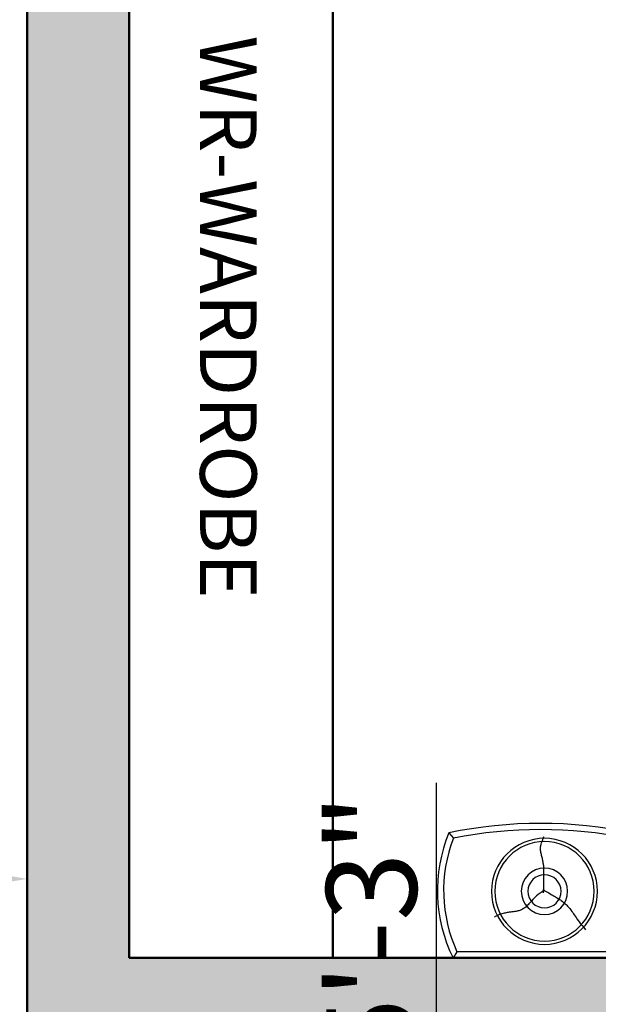
# Model space of a CAD drawing. Units: inches. Extents: x 3008 to 4088, y 1255 to 2137.
# Tile 13 of 30: x 3093 to 3144, y 1787 to 1874. Entities that reach past the tile are written whole.
import ezdxf

# ---------------------------------------------------------------- set-up
doc = ezdxf.new("R2010")
doc.units = ezdxf.units.IN
for name, color, linetype, lineweight in [('A-ANNO-DIMS', 2, 'Continuous', 18), ('A-ANNO-TEXT', 7, 'Continuous', 18), ('A-FURN', 8, 'Continuous', 18), ('A-WALL', 7, 'Continuous', 50), ('A-WALL-PATT', 8, 'Continuous', 13)]:
    doc.layers.add(name, color=color, linetype=linetype, lineweight=lineweight)
doc.layers.add('TEFRİŞ', color=11, linetype='Continuous')
doc.styles.get("Standard").update_dxf_attribs({"font": 'arial.ttf'})
doc.dimstyles.new('ISO-25', dxfattribs={"dimtxt": 8, "dimasz": 2.5, "dimexe": 1.25, "dimexo": 0.625, "dimtad": 1, "dimdec": 1, "dimlunit": 3, "dimtxsty": 'Standard', "dimcen": 2.5, "dimadec": 0, "dimazin": 0, "dimtfac": 1, "dimtdec": 1, "dimtmove": 0, "dimatfit": 3, "dimfxl": 1, "dimarcsym": 0})

# ---------------------------------------------------------------- blocks, each defined once
blk = doc.blocks.new('*D3')
at = {"layer": 'A-ANNO-DIMS', "color": 0, "lineweight": -2, "transparency": 16777216}
for p, q in [((3039.666, 1798.574), (3039.666, 1799.199)), ((3093.666, 1798.574), (3093.666, 1799.199)), ((3042.166, 1797.949), (3091.166, 1797.949))]:
    blk.add_line(p, q, dxfattribs=at)
at = {"layer": 'A-ANNO-DIMS', "color": 0, "transparency": 16777216}
for points in [[(3042.166, 1798.366), (3042.166, 1797.532), (3039.666, 1797.949)], [(3091.166, 1798.366), (3091.166, 1797.532), (3093.666, 1797.949)]]:
    blk.add_solid(points, dxfattribs=at)
at = {"layer": 'Defpoints', "color": 0, "transparency": 16777216}
for p in [(3039.666, 1797.949), (3093.666, 1797.949), (3093.666, 1797.949)]:
    blk.add_point(p, dxfattribs=at)
at = {"layer": 'A-ANNO-DIMS', "color": 0, "transparency": 16777216, "insert": (3066.666, 1802.659), "char_height": 8, "attachment_point": 5}
blk.add_mtext('4\'-6"', dxfattribs=at)
blk = doc.blocks.new('BED')
at = {"layer": 'TEFRİŞ'}
for p, q in [((2177.285, 1835.981), (2177.607, 1835.472)), ((2177.285, 1835.981), (2191.525, 1835.981)), ((2191.203, 1835.472), (2191.525, 1835.981)), ((2114.88, 1835.661), (2129.119, 1835.661)), ((2115.201, 1835.152), (2128.798, 1835.152)), ((2130.81, 1834.338), (2130.81, 1835.55)), ((2130.91, 1835.55), (2175.558, 1835.55)), ((2175.558, 1835.55), (2175.558, 1834.338)), ((2177.607, 1835.472), (2191.203, 1835.472)), ((2175.558, 1834.338), (2130.81, 1834.338)), ((2175.003, 1834.192), (2130.91, 1834.192)), ((2180.9, 1833.519), (2180.747, 1833.698)), ((2180.9, 1833.519), (2180.747, 1833.698)), ((2181.036, 1833.353), (2180.9, 1833.519)), ((2181.036, 1833.353), (2180.9, 1833.519)), ((2118.495, 1833.199), (2118.341, 1833.378)), ((2118.495, 1833.199), (2118.341, 1833.378)), ((2118.631, 1833.033), (2118.495, 1833.199)), ((2118.631, 1833.033), (2118.495, 1833.199)), ((2118.751, 1832.88), (2118.631, 1833.033)), ((2118.751, 1832.88), (2118.631, 1833.033)), ((2118.857, 1832.738), (2118.751, 1832.88)), ((2118.857, 1832.738), (2118.751, 1832.88)), ((2118.952, 1832.606), (2118.857, 1832.738)), ((2118.952, 1832.606), (2118.857, 1832.738)), ((2119.038, 1832.483), (2118.952, 1832.606)), ((2119.038, 1832.483), (2118.952, 1832.606)), ((2181.156, 1833.2), (2181.036, 1833.353)), ((2181.156, 1833.2), (2181.036, 1833.353)), ((2181.263, 1833.058), (2181.156, 1833.2)), ((2181.263, 1833.058), (2181.156, 1833.2)), ((2181.358, 1832.926), (2181.263, 1833.058)), ((2181.358, 1832.926), (2181.263, 1833.058)), ((2181.443, 1832.803), (2181.358, 1832.926)), ((2181.443, 1832.803), (2181.358, 1832.926)), ((2181.521, 1832.688), (2181.443, 1832.803)), ((2181.521, 1832.688), (2181.443, 1832.803)), ((2181.594, 1832.581), (2181.521, 1832.688)), ((2181.594, 1832.581), (2181.521, 1832.688)), ((2188.007, 1832.575), (2188.085, 1832.621)), ((2188.007, 1832.575), (2188.085, 1832.621)), ((2188.085, 1832.621), (2188.155, 1832.67)), ((2188.085, 1832.621), (2188.155, 1832.67)), ((2119.116, 1832.368), (2119.038, 1832.483)), ((2119.116, 1832.368), (2119.038, 1832.483)), ((2119.188, 1832.261), (2119.116, 1832.368)), ((2119.188, 1832.261), (2119.116, 1832.368)), ((2119.257, 1832.159), (2119.188, 1832.261)), ((2119.257, 1832.159), (2119.188, 1832.261)), ((2119.324, 1832.064), (2119.257, 1832.159)), ((2119.324, 1832.064), (2119.257, 1832.159)), ((2119.387, 1831.973), (2119.324, 1832.064)), ((2119.387, 1831.973), (2119.324, 1832.064)), ((2119.449, 1831.887), (2119.387, 1831.973)), ((2119.449, 1831.887), (2119.387, 1831.973)), ((2119.51, 1831.805), (2119.449, 1831.887)), ((2119.51, 1831.805), (2119.449, 1831.887)), ((2119.569, 1831.727), (2119.51, 1831.805)), ((2119.569, 1831.727), (2119.51, 1831.805)), ((2123.622, 1831.774), (2123.693, 1831.8)), ((2123.622, 1831.774), (2123.693, 1831.8)), ((2123.693, 1831.8), (2123.766, 1831.823)), ((2123.693, 1831.8), (2123.766, 1831.823)), ((2123.766, 1831.823), (2123.838, 1831.843)), ((2123.766, 1831.823), (2123.838, 1831.843)), ((2123.838, 1831.843), (2123.911, 1831.86)), ((2123.838, 1831.843), (2123.911, 1831.86)), ((2123.911, 1831.86), (2123.983, 1831.874)), ((2123.911, 1831.86), (2123.983, 1831.874)), ((2123.983, 1831.874), (2124.056, 1831.886)), ((2123.983, 1831.874), (2124.056, 1831.886)), ((2124.056, 1831.886), (2124.128, 1831.896)), ((2124.056, 1831.886), (2124.128, 1831.896)), ((2124.128, 1831.896), (2124.201, 1831.906)), ((2124.128, 1831.896), (2124.201, 1831.906)), ((2124.201, 1831.906), (2124.273, 1831.914)), ((2124.201, 1831.906), (2124.273, 1831.914)), ((2124.273, 1831.914), (2124.346, 1831.923)), ((2124.273, 1831.914), (2124.346, 1831.923)), ((2124.346, 1831.923), (2124.418, 1831.932)), ((2124.346, 1831.923), (2124.418, 1831.932)), ((2124.418, 1831.932), (2124.491, 1831.941)), ((2124.418, 1831.932), (2124.491, 1831.941)), ((2124.491, 1831.941), (2124.564, 1831.952)), ((2124.491, 1831.941), (2124.564, 1831.952)), ((2124.564, 1831.952), (2124.638, 1831.963)), ((2124.564, 1831.952), (2124.638, 1831.963)), ((2124.638, 1831.963), (2124.714, 1831.977)), ((2124.638, 1831.963), (2124.714, 1831.977)), ((2124.714, 1831.977), (2124.793, 1831.992)), ((2124.714, 1831.977), (2124.793, 1831.992)), ((2124.793, 1831.992), (2124.874, 1832.01)), ((2124.793, 1831.992), (2124.874, 1832.01)), ((2124.874, 1832.01), (2124.958, 1832.03)), ((2124.874, 1832.01), (2124.958, 1832.03)), ((2124.958, 1832.03), (2125.047, 1832.052)), ((2124.958, 1832.03), (2125.047, 1832.052)), ((2125.047, 1832.052), (2125.139, 1832.078)), ((2125.047, 1832.052), (2125.139, 1832.078)), ((2125.139, 1832.078), (2125.234, 1832.107)), ((2125.139, 1832.078), (2125.234, 1832.107)), ((2125.234, 1832.107), (2125.33, 1832.139)), ((2125.234, 1832.107), (2125.33, 1832.139)), ((2125.33, 1832.139), (2125.424, 1832.174)), ((2125.33, 1832.139), (2125.424, 1832.174)), ((2125.424, 1832.174), (2125.515, 1832.213)), ((2125.424, 1832.174), (2125.515, 1832.213)), ((2125.515, 1832.213), (2125.601, 1832.255)), ((2125.515, 1832.213), (2125.601, 1832.255)), ((2125.601, 1832.255), (2125.68, 1832.301)), ((2125.601, 1832.255), (2125.68, 1832.301)), ((2125.68, 1832.301), (2125.749, 1832.35)), ((2125.68, 1832.301), (2125.749, 1832.35)), ((2181.663, 1832.479), (2181.594, 1832.581)), ((2181.663, 1832.479), (2181.594, 1832.581)), ((2181.729, 1832.384), (2181.663, 1832.479)), ((2181.729, 1832.384), (2181.663, 1832.479)), ((2181.793, 1832.293), (2181.729, 1832.384)), ((2181.793, 1832.293), (2181.729, 1832.384)), ((2181.855, 1832.207), (2181.793, 1832.293)), ((2181.855, 1832.207), (2181.793, 1832.293)), ((2181.915, 1832.125), (2181.855, 1832.207)), ((2181.915, 1832.125), (2181.855, 1832.207)), ((2181.975, 1832.047), (2181.915, 1832.125)), ((2181.975, 1832.047), (2181.915, 1832.125)), ((2182.034, 1831.972), (2181.975, 1832.047)), ((2182.034, 1831.972), (2181.975, 1832.047)), ((2182.093, 1831.9), (2182.034, 1831.972)), ((2182.093, 1831.9), (2182.034, 1831.972)), ((2182.152, 1831.83), (2182.093, 1831.9)), ((2182.152, 1831.83), (2182.093, 1831.9)), ((2182.212, 1831.762), (2182.152, 1831.83)), ((2182.212, 1831.762), (2182.152, 1831.83)), ((2185.549, 1831.784), (2185.614, 1831.843)), ((2185.549, 1831.784), (2185.614, 1831.843)), ((2185.614, 1831.843), (2185.68, 1831.897)), ((2185.614, 1831.843), (2185.68, 1831.897)), ((2185.68, 1831.897), (2185.747, 1831.946)), ((2185.68, 1831.897), (2185.747, 1831.946)), ((2185.747, 1831.946), (2185.816, 1831.99)), ((2185.747, 1831.946), (2185.816, 1831.99)), ((2185.816, 1831.99), (2185.885, 1832.029)), ((2185.816, 1831.99), (2185.885, 1832.029)), ((2185.885, 1832.029), (2185.956, 1832.063)), ((2185.885, 1832.029), (2185.956, 1832.063)), ((2185.956, 1832.063), (2186.027, 1832.094)), ((2185.956, 1832.063), (2186.027, 1832.094)), ((2186.027, 1832.094), (2186.099, 1832.12)), ((2186.027, 1832.094), (2186.099, 1832.12)), ((2186.099, 1832.12), (2186.171, 1832.143)), ((2186.099, 1832.12), (2186.171, 1832.143)), ((2186.171, 1832.143), (2186.244, 1832.163)), ((2186.171, 1832.143), (2186.244, 1832.163)), ((2186.244, 1832.163), (2186.316, 1832.18)), ((2186.244, 1832.163), (2186.316, 1832.18)), ((2186.316, 1832.18), (2186.389, 1832.194)), ((2186.316, 1832.18), (2186.389, 1832.194)), ((2186.389, 1832.194), (2186.461, 1832.206)), ((2186.389, 1832.194), (2186.461, 1832.206)), ((2186.461, 1832.206), (2186.534, 1832.216)), ((2186.461, 1832.206), (2186.534, 1832.216)), ((2186.534, 1832.216), (2186.606, 1832.226)), ((2186.534, 1832.216), (2186.606, 1832.226)), ((2186.606, 1832.226), (2186.679, 1832.234)), ((2186.606, 1832.226), (2186.679, 1832.234)), ((2186.679, 1832.234), (2186.751, 1832.243)), ((2186.679, 1832.234), (2186.751, 1832.243)), ((2186.751, 1832.243), (2186.824, 1832.252)), ((2186.751, 1832.243), (2186.824, 1832.252)), ((2186.824, 1832.252), (2186.896, 1832.261)), ((2186.824, 1832.252), (2186.896, 1832.261)), ((2186.896, 1832.261), (2186.97, 1832.272)), ((2186.896, 1832.261), (2186.97, 1832.272)), ((2186.97, 1832.272), (2187.044, 1832.283)), ((2186.97, 1832.272), (2187.044, 1832.283)), ((2187.044, 1832.283), (2187.12, 1832.297)), ((2187.044, 1832.283), (2187.12, 1832.297)), ((2187.12, 1832.297), (2187.198, 1832.312)), ((2187.12, 1832.297), (2187.198, 1832.312)), ((2187.198, 1832.312), (2187.279, 1832.33)), ((2187.198, 1832.312), (2187.279, 1832.33)), ((2187.279, 1832.33), (2187.364, 1832.35)), ((2187.279, 1832.33), (2187.364, 1832.35)), ((2187.364, 1832.35), (2187.452, 1832.372)), ((2187.364, 1832.35), (2187.452, 1832.372)), ((2187.452, 1832.372), (2187.545, 1832.398)), ((2187.452, 1832.372), (2187.545, 1832.398)), ((2187.545, 1832.398), (2187.64, 1832.427)), ((2187.545, 1832.398), (2187.64, 1832.427)), ((2187.64, 1832.427), (2187.736, 1832.459)), ((2187.64, 1832.427), (2187.736, 1832.459)), ((2187.736, 1832.459), (2187.83, 1832.494)), ((2187.736, 1832.459), (2187.83, 1832.494)), ((2187.83, 1832.494), (2187.921, 1832.533)), ((2187.83, 1832.494), (2187.921, 1832.533)), ((2187.921, 1832.533), (2188.007, 1832.575)), ((2187.921, 1832.533), (2188.007, 1832.575)), ((2119.628, 1831.652), (2119.569, 1831.727)), ((2119.628, 1831.652), (2119.569, 1831.727)), ((2119.687, 1831.58), (2119.628, 1831.652)), ((2119.687, 1831.58), (2119.628, 1831.652)), ((2119.747, 1831.51), (2119.687, 1831.58)), ((2119.747, 1831.51), (2119.687, 1831.58)), ((2119.807, 1831.442), (2119.747, 1831.51)), ((2119.807, 1831.442), (2119.747, 1831.51)), ((2119.867, 1831.377), (2119.807, 1831.442)), ((2119.867, 1831.377), (2119.807, 1831.442)), ((2119.929, 1831.314), (2119.867, 1831.377)), ((2119.929, 1831.314), (2119.867, 1831.377)), ((2119.991, 1831.254), (2119.929, 1831.314)), ((2119.991, 1831.254), (2119.929, 1831.314)), ((2120.054, 1831.196), (2119.991, 1831.254)), ((2120.054, 1831.196), (2119.991, 1831.254)), ((2120.119, 1831.141), (2120.054, 1831.196)), ((2120.119, 1831.141), (2120.054, 1831.196)), ((2120.185, 1831.088), (2120.119, 1831.141)), ((2120.185, 1831.088), (2120.119, 1831.141)), ((2120.252, 1831.039), (2120.185, 1831.088)), ((2120.252, 1831.039), (2120.185, 1831.088)), ((2120.321, 1830.991), (2120.252, 1831.039)), ((2120.321, 1830.991), (2120.252, 1831.039)), ((2120.392, 1830.944), (2120.321, 1830.991)), ((2120.392, 1830.944), (2120.321, 1830.991)), ((2122.64, 1830.913), (2122.723, 1831.006)), ((2122.64, 1830.913), (2122.723, 1831.006)), ((2122.723, 1831.006), (2122.8, 1831.094)), ((2122.723, 1831.006), (2122.8, 1831.094)), ((2122.8, 1831.094), (2122.874, 1831.178)), ((2122.8, 1831.094), (2122.874, 1831.178)), ((2122.874, 1831.178), (2122.944, 1831.256)), ((2122.874, 1831.178), (2122.944, 1831.256)), ((2122.944, 1831.256), (2123.012, 1831.331)), ((2122.944, 1831.256), (2123.012, 1831.331)), ((2123.012, 1831.331), (2123.078, 1831.4)), ((2123.012, 1831.331), (2123.078, 1831.4)), ((2123.078, 1831.4), (2123.143, 1831.464)), ((2123.078, 1831.4), (2123.143, 1831.464)), ((2123.143, 1831.464), (2123.208, 1831.523)), ((2123.143, 1831.464), (2123.208, 1831.523)), ((2123.208, 1831.523), (2123.274, 1831.577)), ((2123.208, 1831.523), (2123.274, 1831.577)), ((2123.274, 1831.577), (2123.342, 1831.626)), ((2123.274, 1831.577), (2123.342, 1831.626)), ((2123.342, 1831.626), (2123.41, 1831.67)), ((2123.342, 1831.626), (2123.41, 1831.67)), ((2123.41, 1831.67), (2123.48, 1831.709)), ((2123.41, 1831.67), (2123.48, 1831.709)), ((2123.48, 1831.709), (2123.55, 1831.743)), ((2123.48, 1831.709), (2123.55, 1831.743)), ((2123.55, 1831.743), (2123.622, 1831.774)), ((2123.55, 1831.743), (2123.622, 1831.774)), ((2182.273, 1831.697), (2182.212, 1831.762)), ((2182.273, 1831.697), (2182.212, 1831.762)), ((2182.334, 1831.634), (2182.273, 1831.697)), ((2182.334, 1831.634), (2182.273, 1831.697)), ((2182.397, 1831.574), (2182.334, 1831.634)), ((2182.397, 1831.574), (2182.334, 1831.634)), ((2182.46, 1831.516), (2182.397, 1831.574)), ((2182.46, 1831.516), (2182.397, 1831.574)), ((2182.525, 1831.461), (2182.46, 1831.516)), ((2182.525, 1831.461), (2182.46, 1831.516)), ((2182.59, 1831.408), (2182.525, 1831.461)), ((2182.59, 1831.408), (2182.525, 1831.461)), ((2182.658, 1831.359), (2182.59, 1831.408)), ((2182.658, 1831.359), (2182.59, 1831.408)), ((2182.726, 1831.311), (2182.658, 1831.359)), ((2182.726, 1831.311), (2182.658, 1831.359)), ((2182.797, 1831.264), (2182.726, 1831.311)), ((2182.797, 1831.264), (2182.726, 1831.311)), ((2182.871, 1831.218), (2182.797, 1831.264)), ((2182.871, 1831.218), (2182.797, 1831.264)), ((2182.947, 1831.172), (2182.871, 1831.218)), ((2182.947, 1831.172), (2182.871, 1831.218)), ((2183.027, 1831.124), (2182.947, 1831.172)), ((2183.027, 1831.124), (2182.947, 1831.172)), ((2183.11, 1831.074), (2183.027, 1831.124)), ((2183.11, 1831.074), (2183.027, 1831.124)), ((2183.196, 1831.022), (2183.11, 1831.074)), ((2183.196, 1831.022), (2183.11, 1831.074)), ((2183.288, 1830.966), (2183.196, 1831.022)), ((2183.288, 1830.966), (2183.196, 1831.022)), ((2184.736, 1830.933), (2184.852, 1831.036)), ((2184.736, 1830.933), (2184.852, 1831.036)), ((2184.852, 1831.036), (2184.954, 1831.136)), ((2184.852, 1831.036), (2184.954, 1831.136)), ((2184.954, 1831.136), (2185.045, 1831.233)), ((2184.954, 1831.136), (2185.045, 1831.233)), ((2185.045, 1831.233), (2185.128, 1831.326)), ((2185.045, 1831.233), (2185.128, 1831.326)), ((2185.128, 1831.326), (2185.206, 1831.414)), ((2185.128, 1831.326), (2185.206, 1831.414)), ((2185.206, 1831.414), (2185.279, 1831.498)), ((2185.206, 1831.414), (2185.279, 1831.498)), ((2185.279, 1831.498), (2185.35, 1831.577)), ((2185.279, 1831.498), (2185.35, 1831.577)), ((2185.35, 1831.577), (2185.418, 1831.651)), ((2185.35, 1831.577), (2185.418, 1831.651)), ((2185.418, 1831.651), (2185.484, 1831.72)), ((2185.418, 1831.651), (2185.484, 1831.72)), ((2185.484, 1831.72), (2185.549, 1831.784)), ((2185.484, 1831.72), (2185.549, 1831.784)), ((2120.465, 1830.898), (2120.392, 1830.944)), ((2120.465, 1830.898), (2120.392, 1830.944)), ((2120.542, 1830.852), (2120.465, 1830.898)), ((2120.542, 1830.852), (2120.465, 1830.898)), ((2120.621, 1830.804), (2120.542, 1830.852)), ((2120.621, 1830.804), (2120.542, 1830.852)), ((2120.704, 1830.754), (2120.621, 1830.804)), ((2120.704, 1830.754), (2120.621, 1830.804)), ((2120.791, 1830.702), (2120.704, 1830.754)), ((2120.791, 1830.702), (2120.704, 1830.754)), ((2120.882, 1830.646), (2120.791, 1830.702)), ((2120.882, 1830.646), (2120.791, 1830.702)), ((2120.98, 1830.585), (2120.882, 1830.646)), ((2120.98, 1830.585), (2120.882, 1830.646)), ((2121.088, 1830.521), (2120.98, 1830.585)), ((2121.088, 1830.521), (2120.98, 1830.585)), ((2121.207, 1830.451), (2121.088, 1830.521)), ((2121.207, 1830.451), (2121.088, 1830.521)), ((2121.34, 1830.376), (2121.207, 1830.451)), ((2121.34, 1830.376), (2121.207, 1830.451)), ((2121.489, 1830.295), (2121.34, 1830.376)), ((2121.489, 1830.295), (2121.34, 1830.376)), ((2121.658, 1830.207), (2121.489, 1830.295)), ((2121.658, 1830.207), (2121.489, 1830.295)), ((2121.848, 1830.113), (2121.658, 1830.207)), ((2121.848, 1830.113), (2121.658, 1830.207)), ((2121.663, 1830.184), (2121.867, 1830.293)), ((2121.663, 1830.184), (2121.867, 1830.293)), ((2121.76, 1830.377), (2121.745, 1830.173)), ((2121.76, 1830.377), (2121.745, 1830.173)), ((2121.867, 1830.293), (2122.043, 1830.401)), ((2121.867, 1830.293), (2122.043, 1830.401)), ((2122.043, 1830.401), (2122.197, 1830.508)), ((2122.043, 1830.401), (2122.197, 1830.508)), ((2122.197, 1830.508), (2122.33, 1830.613)), ((2122.197, 1830.508), (2122.33, 1830.613)), ((2122.33, 1830.613), (2122.446, 1830.716)), ((2122.33, 1830.613), (2122.446, 1830.716)), ((2122.446, 1830.716), (2122.549, 1830.816)), ((2122.446, 1830.716), (2122.549, 1830.816)), ((2122.549, 1830.816), (2122.64, 1830.913)), ((2122.549, 1830.816), (2122.64, 1830.913)), ((2183.386, 1830.905), (2183.288, 1830.966)), ((2183.386, 1830.905), (2183.288, 1830.966)), ((2183.493, 1830.841), (2183.386, 1830.905)), ((2183.493, 1830.841), (2183.386, 1830.905)), ((2183.612, 1830.771), (2183.493, 1830.841)), ((2183.612, 1830.771), (2183.493, 1830.841)), ((2183.745, 1830.696), (2183.612, 1830.771)), ((2183.745, 1830.696), (2183.612, 1830.771)), ((2183.895, 1830.615), (2183.745, 1830.696)), ((2183.895, 1830.615), (2183.745, 1830.696)), ((2184.064, 1830.527), (2183.895, 1830.615)), ((2184.064, 1830.527), (2183.895, 1830.615)), ((2184.254, 1830.433), (2184.064, 1830.527)), ((2184.254, 1830.433), (2184.064, 1830.527)), ((2184.069, 1830.504), (2184.272, 1830.613)), ((2184.069, 1830.504), (2184.272, 1830.613)), ((2184.141, 1830.313), (2184.137, 1830.154)), ((2184.141, 1830.313), (2184.137, 1830.154)), ((2184.151, 1830.493), (2184.141, 1830.313)), ((2184.151, 1830.493), (2184.141, 1830.313)), ((2184.165, 1830.697), (2184.151, 1830.493)), ((2184.165, 1830.697), (2184.151, 1830.493)), ((2184.272, 1830.613), (2184.449, 1830.721)), ((2184.272, 1830.613), (2184.449, 1830.721)), ((2184.449, 1830.721), (2184.603, 1830.828)), ((2184.449, 1830.721), (2184.603, 1830.828)), ((2184.603, 1830.828), (2184.736, 1830.933)), ((2184.603, 1830.828), (2184.736, 1830.933)), ((2121.731, 1829.834), (2121.73, 1829.693)), ((2121.731, 1829.834), (2121.73, 1829.693)), ((2121.73, 1829.693), (2121.732, 1829.567)), ((2121.73, 1829.693), (2121.732, 1829.567)), ((2121.736, 1829.993), (2121.731, 1829.834)), ((2121.736, 1829.993), (2121.731, 1829.834)), ((2121.732, 1829.567), (2121.734, 1829.453)), ((2121.732, 1829.567), (2121.734, 1829.453)), ((2121.734, 1829.453), (2121.737, 1829.349)), ((2121.734, 1829.453), (2121.737, 1829.349)), ((2121.745, 1830.173), (2121.736, 1829.993)), ((2121.745, 1830.173), (2121.736, 1829.993)), ((2184.137, 1830.154), (2184.136, 1830.013)), ((2184.137, 1830.154), (2184.136, 1830.013)), ((2184.136, 1830.013), (2184.137, 1829.887)), ((2184.136, 1830.013), (2184.137, 1829.887)), ((2184.137, 1829.887), (2184.14, 1829.773)), ((2184.137, 1829.887), (2184.14, 1829.773)), ((2184.14, 1829.773), (2184.143, 1829.669)), ((2184.14, 1829.773), (2184.143, 1829.669)), ((2184.143, 1829.669), (2184.145, 1829.57)), ((2184.143, 1829.669), (2184.145, 1829.57)), ((2184.145, 1829.57), (2184.146, 1829.475)), ((2184.145, 1829.57), (2184.146, 1829.475)), ((2184.146, 1829.475), (2184.145, 1829.383)), ((2184.146, 1829.475), (2184.145, 1829.383)), ((2121.73, 1828.718), (2121.728, 1828.637)), ((2121.73, 1828.718), (2121.728, 1828.637)), ((2121.728, 1828.637), (2121.728, 1828.558)), ((2121.728, 1828.637), (2121.728, 1828.558)), ((2121.733, 1828.801), (2121.73, 1828.718)), ((2121.733, 1828.801), (2121.73, 1828.718)), ((2121.735, 1828.886), (2121.733, 1828.801)), ((2121.735, 1828.886), (2121.733, 1828.801)), ((2121.738, 1828.973), (2121.735, 1828.886)), ((2121.738, 1828.973), (2121.735, 1828.886)), ((2121.737, 1829.349), (2121.74, 1829.25)), ((2121.737, 1829.349), (2121.74, 1829.25)), ((2121.74, 1829.063), (2121.738, 1828.973)), ((2121.74, 1829.063), (2121.738, 1828.973)), ((2121.74, 1829.25), (2121.74, 1829.155)), ((2121.74, 1829.25), (2121.74, 1829.155)), ((2121.74, 1829.155), (2121.74, 1829.063)), ((2121.74, 1829.155), (2121.74, 1829.063)), ((2184.134, 1828.957), (2184.133, 1828.878)), ((2184.134, 1828.957), (2184.133, 1828.878)), ((2184.133, 1828.878), (2184.134, 1828.8)), ((2184.133, 1828.878), (2184.134, 1828.8)), ((2184.136, 1829.038), (2184.134, 1828.957)), ((2184.136, 1829.038), (2184.134, 1828.957)), ((2184.134, 1828.8), (2184.136, 1828.723)), ((2184.134, 1828.8), (2184.136, 1828.723)), ((2184.138, 1829.121), (2184.136, 1829.038)), ((2184.138, 1829.121), (2184.136, 1829.038)), ((2184.136, 1828.723), (2184.14, 1828.648)), ((2184.136, 1828.723), (2184.14, 1828.648)), ((2184.141, 1829.206), (2184.138, 1829.121)), ((2184.141, 1829.206), (2184.138, 1829.121)), ((2184.14, 1828.648), (2184.145, 1828.573)), ((2184.14, 1828.648), (2184.145, 1828.573)), ((2184.143, 1829.293), (2184.141, 1829.206)), ((2184.143, 1829.293), (2184.141, 1829.206)), ((2184.145, 1829.383), (2184.143, 1829.293)), ((2184.145, 1829.383), (2184.143, 1829.293)), ((2121.728, 1828.558), (2121.728, 1828.48)), ((2121.728, 1828.558), (2121.728, 1828.48)), ((2121.728, 1828.48), (2121.731, 1828.403)), ((2121.728, 1828.48), (2121.731, 1828.403)), ((2121.731, 1828.403), (2121.734, 1828.328)), ((2121.731, 1828.403), (2121.734, 1828.328)), ((2121.734, 1828.328), (2121.74, 1828.253)), ((2121.734, 1828.328), (2121.74, 1828.253)), ((2121.74, 1828.253), (2121.747, 1828.178)), ((2121.74, 1828.253), (2121.747, 1828.178)), ((2121.747, 1828.178), (2121.755, 1828.104)), ((2121.747, 1828.178), (2121.755, 1828.104)), ((2121.755, 1828.104), (2121.765, 1828.029)), ((2121.755, 1828.104), (2121.765, 1828.029)), ((2121.765, 1828.029), (2121.776, 1827.954)), ((2121.765, 1828.029), (2121.776, 1827.954)), ((2121.776, 1827.954), (2121.789, 1827.878)), ((2121.776, 1827.954), (2121.789, 1827.878)), ((2121.789, 1827.878), (2121.803, 1827.801)), ((2121.789, 1827.878), (2121.803, 1827.801)), ((2121.803, 1827.801), (2121.819, 1827.724)), ((2121.803, 1827.801), (2121.819, 1827.724)), ((2184.145, 1828.573), (2184.152, 1828.498)), ((2184.145, 1828.573), (2184.152, 1828.498)), ((2184.152, 1828.498), (2184.16, 1828.424)), ((2184.152, 1828.498), (2184.16, 1828.424)), ((2184.16, 1828.424), (2184.17, 1828.349)), ((2184.16, 1828.424), (2184.17, 1828.349)), ((2184.17, 1828.349), (2184.182, 1828.274)), ((2184.17, 1828.349), (2184.182, 1828.274)), ((2184.182, 1828.274), (2184.194, 1828.198)), ((2184.182, 1828.274), (2184.194, 1828.198)), ((2184.194, 1828.198), (2184.209, 1828.121)), ((2184.194, 1828.198), (2184.209, 1828.121)), ((2184.209, 1828.121), (2184.224, 1828.044)), ((2184.209, 1828.121), (2184.224, 1828.044)), ((2184.224, 1828.044), (2184.241, 1827.967)), ((2184.224, 1828.044), (2184.241, 1827.967)), ((2184.241, 1827.967), (2184.259, 1827.889)), ((2184.241, 1827.967), (2184.259, 1827.889)), ((2184.259, 1827.889), (2184.278, 1827.811)), ((2184.259, 1827.889), (2184.278, 1827.811)), ((2184.278, 1827.811), (2184.298, 1827.732)), ((2184.278, 1827.811), (2184.298, 1827.732)), ((2121.819, 1827.724), (2121.835, 1827.647)), ((2121.819, 1827.724), (2121.835, 1827.647)), ((2121.835, 1827.647), (2121.853, 1827.569)), ((2121.835, 1827.647), (2121.853, 1827.569)), ((2121.853, 1827.569), (2121.872, 1827.491)), ((2121.853, 1827.569), (2121.872, 1827.491)), ((2121.872, 1827.491), (2121.892, 1827.412)), ((2121.872, 1827.491), (2121.892, 1827.412)), ((2121.892, 1827.412), (2121.913, 1827.334)), ((2121.892, 1827.412), (2121.913, 1827.334)), ((2121.913, 1827.334), (2121.934, 1827.255)), ((2121.913, 1827.334), (2121.934, 1827.255)), ((2121.934, 1827.255), (2121.955, 1827.176)), ((2121.934, 1827.255), (2121.955, 1827.176)), ((2121.955, 1827.176), (2121.974, 1827.095)), ((2121.955, 1827.176), (2121.974, 1827.095)), ((2121.974, 1827.095), (2121.989, 1827.012)), ((2121.974, 1827.095), (2121.989, 1827.012)), ((2121.989, 1827.012), (2122.001, 1826.925)), ((2121.989, 1827.012), (2122.001, 1826.925)), ((2184.298, 1827.732), (2184.319, 1827.654)), ((2184.298, 1827.732), (2184.319, 1827.654)), ((2184.319, 1827.654), (2184.34, 1827.575)), ((2184.319, 1827.654), (2184.34, 1827.575)), ((2184.34, 1827.575), (2184.361, 1827.496)), ((2184.34, 1827.575), (2184.361, 1827.496)), ((2184.361, 1827.496), (2184.379, 1827.415)), ((2184.361, 1827.496), (2184.379, 1827.415)), ((2184.379, 1827.415), (2184.395, 1827.332)), ((2184.379, 1827.415), (2184.395, 1827.332)), ((2184.395, 1827.332), (2184.406, 1827.245)), ((2184.395, 1827.332), (2184.406, 1827.245)), ((2184.409, 1827.061), (2184.399, 1826.961)), ((2184.409, 1827.061), (2184.399, 1826.961)), ((2184.406, 1827.245), (2184.411, 1827.156)), ((2184.406, 1827.245), (2184.411, 1827.156)), ((2184.411, 1827.156), (2184.409, 1827.061)), ((2184.411, 1827.156), (2184.409, 1827.061)), ((2121.872, 1826.187), (2121.829, 1826.062)), ((2121.872, 1826.187), (2121.829, 1826.062)), ((2121.911, 1826.308), (2121.872, 1826.187)), ((2121.911, 1826.308), (2121.872, 1826.187)), ((2121.946, 1826.424), (2121.911, 1826.308)), ((2121.946, 1826.424), (2121.911, 1826.308)), ((2121.974, 1826.536), (2121.946, 1826.424)), ((2121.974, 1826.536), (2121.946, 1826.424)), ((2121.994, 1826.641), (2121.974, 1826.536)), ((2121.994, 1826.641), (2121.974, 1826.536)), ((2122.004, 1826.741), (2121.994, 1826.641)), ((2122.004, 1826.741), (2121.994, 1826.641)), ((2122.001, 1826.925), (2122.006, 1826.835)), ((2122.001, 1826.925), (2122.006, 1826.835)), ((2122.006, 1826.835), (2122.004, 1826.741)), ((2122.006, 1826.835), (2122.004, 1826.741)), ((2176.942, 1825.81), (2177.313, 1826.253)), ((2184.19, 1826.253), (2184.145, 1826.12)), ((2184.19, 1826.253), (2184.145, 1826.12)), ((2184.234, 1826.382), (2184.19, 1826.253)), ((2184.234, 1826.382), (2184.19, 1826.253)), ((2184.277, 1826.507), (2184.234, 1826.382)), ((2184.277, 1826.507), (2184.234, 1826.382)), ((2184.317, 1826.628), (2184.277, 1826.507)), ((2184.317, 1826.628), (2184.277, 1826.507)), ((2184.351, 1826.744), (2184.317, 1826.628)), ((2184.351, 1826.744), (2184.317, 1826.628)), ((2184.379, 1826.856), (2184.351, 1826.744)), ((2184.379, 1826.856), (2184.351, 1826.744)), ((2184.399, 1826.961), (2184.379, 1826.856)), ((2184.399, 1826.961), (2184.379, 1826.856)), ((2191.868, 1825.81), (2191.497, 1826.253)), ((2121.784, 1825.933), (2121.739, 1825.8)), ((2121.784, 1825.933), (2121.739, 1825.8)), ((2121.829, 1826.062), (2121.784, 1825.933)), ((2121.829, 1826.062), (2121.784, 1825.933)), ((2129.463, 1825.49), (2129.092, 1825.933)), ((2174.766, 1820.529), (2130.76, 1800.908)), ((2174.766, 1819.766), (2130.596, 1795.832)), ((2140.432, 1818.692), (2131.535, 1818.692)), ((2157.712, 1818.692), (2156.771, 1818.692)), ((2170.414, 1818.692), (2164.917, 1818.692)), ((2141.428, 1817.4), (2131.53, 1817.4)), ((2149.625, 1817.4), (2145.875, 1817.4)), ((2167.356, 1817.4), (2154.767, 1817.4)), ((2175.003, 1776.572), (2130.11, 1776.572)), ((2138.519, 1775.41), (2167.387, 1775.41))]:
    blk.add_line(p, q, dxfattribs=at)
for centre, radius, start, end in [((2188.403, 1830.514), 12.389, 153.81622, 202.31399), ((2180.407, 1830.514), 12.389, 337.68603, 26.18379), ((2125.998, 1830.194), 12.389, 153.81622, 202.31399), ((2125.998, 1830.194), 11.881, 155.33353, 201.01573), ((2118.001, 1830.194), 11.881, 338.98429, 24.66649), ((2118.001, 1830.194), 12.389, 337.68603, 26.18379), ((2188.403, 1830.514), 11.881, 155.33353, 201.01573), ((2180.407, 1830.514), 11.881, 338.98429, 24.66649), ((2184.405, 1861.673), 36.123, 258.67732, 281.32269), ((2121.999, 1861.353), 36.631, 258.24432, 281.75569), ((2121.999, 1861.353), 36.123, 258.67732, 281.32269), ((2184.405, 1861.673), 36.631, 258.24432, 281.75569)]:
    blk.add_arc(centre, radius, start, end, dxfattribs=at)
at = {"layer": 'TEFRİŞ', "extrusion": (0, 0, -1)}
for centre, major_axis, ratio, start_param, end_param in [((2121.682, 1830.245), (-3.048, -3.048), 1, 3.926991, 10.210176), ((2121.682, 1830.245), (2.857, -2.857), 1, 5.497787, 11.780972), ((2121.682, 1830.245), (2.857, -2.857), 1, 5.497787, 11.780972), ((2206.14, 1830.727), (-52.859, -52.859), 1, 0.767743, 0.83177), ((2138.854, 1803.048), (-22.102, 22.102), 1, 0.544604, 1.006234), ((2154.124, 1796.609), (-26.463, 26.463), 1, 0.596409, 0.940188), ((2167.599, 1797.72), (-0.513, 36.467), 0.865194, -0.185965, 0.185965), ((2184.087, 1830.565), (-3.048, -3.048), 1, 3.926991, 10.210176), ((2184.087, 1830.565), (2.857, -2.857), 1, 5.497787, 11.780972), ((2184.087, 1830.565), (2.857, -2.857), 1, 5.497787, 11.780972), ((2139.426, 1773.835), (-42.352, 42.352), 1, 0.646251, 0.896949), ((2154.703, 1828.889), (-15.681, 15.681), 1, -1.00675, -0.580436), ((2181.608, 1828.445), (-34.394, 34.394), 1, -0.888486, -0.672463), ((2164.514, 1832.79), (-13.41, 13.41), 1, -0.974476, -0.730892), ((2127.599, 1828.811), (-13.23, 13.23), 1, 2.100388, 2.328052), ((2155.001, 1761.9), (-50.654, -50.654), 1, 2.239512, 2.426533), ((2128.438, 1832.957), (-13.261, -13.261), 1, 3.889049, 4.127298), ((2183.72, 1833.217), (-17, 17), 1, -0.967105, -0.749712), ((2134.003, 1828.801), (-18.617, 18.617), 1, 2.173461, 2.355043), ((2168.354, 1789.27), (-1.332, 44.62), 0.875277, -0.163954, 0.163954), ((2199.2, 1828.446), (-27.061, -27.061), 1, 0.770625, 0.917228), ((2087.318, 1833.958), (-52.373, 52.373), 1, 2.358049, 2.431787), ((2164.154, 1828.698), (-6.989, 6.989), 1, 1.789136, 2.946702), ((2156.756, 1828.981), (-11.901, -11.901), 1, 3.646453, 4.226155), ((2099.767, 1830.727), (-52.859, 52.859), 1, 2.311571, 2.373849), ((2172.014, 1828.66), (-17.934, 17.934), 1, -0.753394, -0.598744), ((2121.682, 1830.245), (1.333, -1.333), 1, 5.497787, 11.780972), ((2121.682, 1830.245), (1.333, -1.333), 1, 5.497787, 11.780972), ((2184.087, 1830.565), (1.333, -1.333), 1, 5.497787, 11.780972), ((2184.087, 1830.565), (1.333, -1.333), 1, 5.497787, 11.780972), ((2184.087, 1830.565), (0.952, -0.952), 1, 5.497787, 11.780972), ((2184.087, 1830.565), (0.952, -0.952), 1, 5.497787, 11.780972), ((2121.682, 1830.245), (0.952, -0.952), 1, 5.497787, 11.780972), ((2121.682, 1830.245), (0.952, -0.952), 1, 5.497787, 11.780972), ((2159.554, 1823.326), (-5.808, 5.808), 1, -0.516587, 0.256776), ((2154.836, 1827.746), (-1.933, 1.933), 1, 0.997904, 1.977819), ((2675.38, 1815.09), (-384.786, -384.786), 1, 0.80103, 0.811711), ((2166.672, 1824.957), (-2.925, 3.91), 0.760601, -0.723751, 0.723751), ((2153.876, 1825.055), (-9.219, 9.219), 1, 1.994956, 2.818753), ((1630.527, 1815.09), (-384.786, 384.786), 1, 2.329881, 2.340562), ((2147.435, 1824.405), (-3.356, -3.356), 1, 1.11934, 2.270556), ((2145.656, 1827.006), (-1.616, 1.616), 1, 1.310976, 2.284591), ((2172.001, 1826.443), (-11.234, 11.234), 1, -1.332486, -0.624868), ((2158.817, 1823.552), (-3.743, -3.743), 1, 1.730792, 3.47045), ((2141.713, 1819.829), (-11.857, 11.857), 1, 1.850844, 2.42862), ((2157.833, 1821.534), (-4.466, 4.466), 1, 0.576679, 2.021689), ((2140.05, 1819.864), (-5.101, 5.101), 1, 0.238357, 1.390139), ((2139.423, 1820.794), (-4.212, -4.212), 1, 1.82161, 3.349145), ((2160.605, 1825.982), (-9.679, -9.679), 1, 0.009196, 0.886853), ((2148.351, 1820.653), (-4.632, -4.632), 1, 2.117602, 3.020837), ((2147.859, 1820.636), (-4.475, 4.475), 1, 0.665914, 1.867503), ((2148.154, 1825.25), (-7.137, -7.137), 1, 6.061986, 7.190757), ((2170.679, 1829.674), (-16.786, 16.786), 1, -1.354718, -0.902276), ((2154.93, 1828.476), (-11.955, 11.955), 1, -1.530302, -0.934407), ((2127.374, 1815.764), (-10.678, 10.678), 1, 1.657204, 1.779381), ((2132.425, 1774.088), (-35.409, -35.409), 1, 2.362911, 2.464592), ((2140.172, 1862.956), (-27.986, 27.986), 1, 3.983025, 4.107469), ((2165.734, 1860.689), (-26.411, -26.411), 1, 5.306413, 5.463767), ((2199.625, 1529.474), (-209.203, 209.203), 1, 0.675361, 0.697001), ((2146.083, 1822.571), (-10.496, 10.496), 1, -0.951783, -0.716225), ((2159.823, 1822.571), (-10.496, -10.496), 1, 3.857817, 4.093375), ((2127.374, 1815.764), (-10.678, 10.678), 1, 1.94252, 2.248924), ((2111.061, 1818.117), (-14.483, 14.483), 1, 2.258605, 2.412359), ((2150.792, 1825.179), (-6.002, 6.002), 1, 3.032122, 4.026148), ((2159.024, 1834.895), (-3.043, 16.533), 0.830169, 2.822117, 3.461068), ((2194.846, 1818.117), (-14.483, 14.483), 1, -0.841563, -0.687809), ((2141.331, 1830.48), (-9.551, -9.551), 1, 4.941413, 5.601673), ((2169.923, 1815.006), (-27.197, -27.197), 1, 0.734393, 0.836404), ((2135.984, 1815.006), (-27.197, -27.197), 1, 3.875985, 3.977996), ((2098.243, 1811.675), (-23.543, -23.543), 1, 3.885834, 4.043401), ((2207.663, 1811.675), (-23.543, -23.543), 1, 0.668988, 0.826555), ((2189.033, 1803.74), (-40.915, -40.915), 1, 0.789771, 0.855756), ((2116.874, 1803.74), (-40.915, 40.915), 1, 2.285836, 2.351822), ((2122.144, 1803.626), (-6.388, -6.388), 1, 3.886359, 4.265474), ((2222.764, 1798.775), (-34.161, -34.161), 1, 0.743488, 0.893627), ((2135.018, 1798.413), (-3.453, 3.453), 1, -0.831635, -0.314979), ((2135.475, 1797.998), (-3.775, -3.775), 1, 0.329385, 0.820948), ((2148.064, 1790.382), (-0.752, 67.37), 0.394952, 1.480524, 1.661068), ((2127.762, 1790.227), (-0.996, 12.366), 0.296708, 1.141067, 2.000525), ((2118.494, 1784.203), (-9.24, -9.24), 1, 3.839645, 4.088086), ((2182.268, 1782.993), (-5.519, -5.519), 1, 0.671703, 0.993321), ((2162.122, 1778.86), (-21.849, 21.849), 1, -0.78611, -0.680117), ((2143.785, 1778.86), (-21.849, 21.849), 1, 2.250913, 2.356906), ((2129.828, 1778.803), (-0.986, 0.986), 1, 2.330985, 3.163296), ((2176.079, 1778.803), (-0.986, 0.986), 1, 4.690686, 5.522997), ((2132.724, 1775.917), (-1.905, -1.905), 1, 0.284117, 1.557111), ((2173.183, 1775.917), (-1.905, -1.905), 1, 3.155278, 4.428271), ((2134.732, 1774.064), (-0.964, -0.964), 1, 1.381176, 2.701227), ((2136.747, 1781.143), (-4.244, 4.244), 1, 3.62713, 4.188813), ((2169.16, 1781.143), (-4.244, 4.244), 1, 3.665169, 4.226852), ((2171.174, 1774.064), (-0.964, -0.964), 1, 2.011162, 3.331212), ((2131.788, 1775.277), (-1.11, 1.11), 1, 3.629269, 5.067473), ((2130.834, 1776.997), (-2.488, -2.488), 1, 4.590984, 5.084038), ((2175.073, 1776.997), (-2.488, 2.488), 1, 4.34074, 4.833793), ((2174.119, 1775.277), (-1.11, 1.11), 1, 2.786508, 4.224712)]:
    blk.add_ellipse(centre, major_axis=major_axis, ratio=ratio, start_param=start_param, end_param=end_param, dxfattribs=at)
blk = doc.blocks.new('*D71')
at = {"layer": 'A-ANNO-DIMS', "color": 0, "lineweight": -2, "transparency": 16777216}
for p, q in [((3129.831, 1734.668), (3129.831, 1806.45)), ((3121.007, 1734.668), (3131.081, 1734.668)), ((3129.831, 1674.175), (3129.831, 1732.168)), ((3121.007, 1671.675), (3131.081, 1671.675))]:
    blk.add_line(p, q, dxfattribs=at)
at = {"layer": 'A-ANNO-DIMS', "color": 0, "transparency": 16777216}
for points in [[(3129.414, 1732.168), (3130.248, 1732.168), (3129.831, 1734.668)], [(3129.414, 1674.175), (3130.248, 1674.175), (3129.831, 1671.675)]]:
    blk.add_solid(points, dxfattribs=at)
at = {"layer": 'Defpoints', "color": 0, "transparency": 16777216}
for p in [(3120.382, 1734.668), (3129.831, 1734.668), (3120.382, 1671.675)]:
    blk.add_point(p, dxfattribs=at)
at = {"layer": 'A-ANNO-DIMS', "color": 0, "transparency": 16777216, "insert": (3125.119, 1771.809), "char_height": 8, "attachment_point": 5, "rotation": 90}
blk.add_mtext('TV UNIT 5\'-3"', dxfattribs=at)

msp = doc.modelspace()

# ---------------------------------------------------------------- hatches: boundary and pattern name
at = {"layer": 'A-WALL-PATT'}
h = msp.add_hatch(color=256, dxfattribs=at)
h.dxf.hatch_style = 1
h.paths.add_polyline_path([(3102.666, 1625.966), (3093.666, 1625.966), (3093.666, 1540.966), (3102.666, 1540.966)])
h.paths.add_polyline_path([(3102.666, 1784.966), (3252.666, 1784.966), (3252.666, 1790.966), (3102.666, 1790.966), (3102.666, 1892.966), (3093.666, 1892.966), (3093.666, 1667.966), (3102.666, 1667.966)])
h.paths.add_polyline_path([(3192.666, 1943.966), (3093.666, 1943.966), (3093.666, 1934.966), (3102.666, 1934.966), (3192.666, 1934.966)])
h.paths.add_polyline_path([(3264.666, 1943.966), (3234.666, 1943.966), (3234.666, 1934.966), (3246.666, 1934.966), (3246.666, 1868.966), (3252.666, 1868.966), (3252.666, 1934.966), (3264.666, 1934.966)])
h.paths.add_polyline_path([(3330.666, 1943.966), (3288.666, 1943.966), (3288.666, 1934.966), (3300.666, 1934.966), (3300.666, 1838.966), (3246.666, 1838.966), (3246.666, 1826.966), (3252.666, 1826.966), (3252.666, 1832.966), (3306.666, 1832.966), (3306.666, 1934.966), (3330.666, 1934.966)])
h.paths.add_polyline_path([(3390.666, 1943.966), (3360.666, 1943.966), (3360.666, 1934.966), (3390.666, 1934.966)])
h.paths.add_polyline_path([(3465.666, 1943.966), (3432.666, 1943.966), (3432.666, 1934.966), (3456.666, 1934.966), (3456.666, 1883.966), (3465.666, 1883.966)])
h.paths.add_polyline_path([(3465.666, 1841.966), (3456.666, 1841.966), (3456.666, 1790.966), (3370.666, 1790.966), (3370.666, 1784.966), (3456.666, 1784.966), (3456.666, 1759.466), (3465.666, 1759.466)])
h.paths.add_polyline_path([(3465.666, 1693.466), (3456.666, 1693.466), (3456.666, 1667.966), (3330.666, 1667.966), (3330.666, 1643.966), (3336.666, 1643.966), (3336.666, 1661.966), (3456.666, 1661.966), (3456.666, 1649.966), (3465.666, 1649.966)])
h.paths.add_polyline_path([(3465.666, 1625.966), (3456.666, 1625.966), (3456.666, 1613.966), (3324.666, 1613.966), (3324.666, 1604.966), (3456.666, 1604.966), (3456.666, 1571.966), (3465.666, 1571.966)])
h.paths.add_polyline_path([(3465.666, 1505.966), (3456.666, 1505.966), (3456.666, 1472.966), (3438.666, 1472.966), (3438.666, 1463.966), (3465.666, 1463.966)])
h.paths.add_polyline_path([(3396.666, 1472.966), (3354.666, 1472.966), (3354.666, 1463.966), (3396.666, 1463.966)])
h.paths.add_polyline_path([(3312.666, 1472.966), (3288.666, 1472.966), (3288.666, 1550.966), (3282.666, 1550.966), (3282.666, 1472.966), (3270.666, 1472.966), (3270.666, 1463.966), (3312.666, 1463.966)])
h.paths.add_polyline_path([(3246.666, 1472.966), (3234.666, 1472.966), (3234.666, 1544.966), (3252.666, 1544.966), (3252.666, 1550.966), (3234.666, 1550.966), (3234.666, 1604.966), (3282.666, 1604.966), (3282.666, 1580.966), (3288.666, 1580.966), (3288.666, 1613.966), (3150.666, 1613.966), (3150.666, 1604.966), (3225.666, 1604.966), (3225.666, 1463.966), (3246.666, 1463.966)])

# ---------------------------------------------------------------- linework, layer by layer
at = {"layer": 'A-WALL'}
for p, q in [((3093.666, 1540.966), (3093.666, 1943.966)), ((3102.666, 1790.966), (3102.666, 1934.966)), ((3120.666, 1790.966), (3120.666, 1934.966)), ((3102.666, 1790.966), (3252.666, 1790.966))]:
    msp.add_line(p, q, dxfattribs=at)

# ---------------------------------------------------------------- block references
at = {"layer": 'A-FURN', "xscale": 1.086875874800008, "yscale": 1.086875874800008, "zscale": 1.086875874800008, "rotation": 180}
msp.add_blockref('BED', (5513.206, 3786.449), dxfattribs=at)

# ---------------------------------------------------------------- texts
at = {"layer": 'A-ANNO-TEXT', "insert": (3113.931, 1872.445), "char_height": 5, "attachment_point": 1, "rotation": 270}
msp.add_mtext_dynamic_manual_height_columns('{\\fTimes New Roman|b0|i0|c0|p18;WR-WARDROBE}', width=105.61268, gutter_width=12.5, heights=[0], dxfattribs=at)

# ---------------------------------------------------------------- dimensions: what is measured, and where the dimension line sits
at = {"layer": 'A-ANNO-DIMS'}
dim = msp.add_linear_dim(base=(3093.666, 1797.949), p1=(3039.666, 1797.949), p2=(3093.666, 1797.949), dimstyle='ISO-25', override={"dimclrd": 0, "dimclre": 0, "dimclrt": 0}, dxfattribs=at)
dim.commit()
dim.dimension.update_dxf_attribs({"geometry": '*D3', "text_midpoint": (3066.666, 1802.659)})
dim = msp.add_linear_dim(base=(3129.831, 1734.668), p1=(3120.382, 1671.675), p2=(3120.382, 1734.668), angle=90, text='TV UNIT <>', dimstyle='ISO-25', override={"dimdec": 1, "dimrnd": 0, "dimzin": 1, "dimlunit": 4, "dimfrac": 2}, dxfattribs=at)
dim.commit()
dim.dimension.update_dxf_attribs({"geometry": '*D71', "text_midpoint": (3125.119, 1771.809)})

doc.saveas('drawing.dxf')
